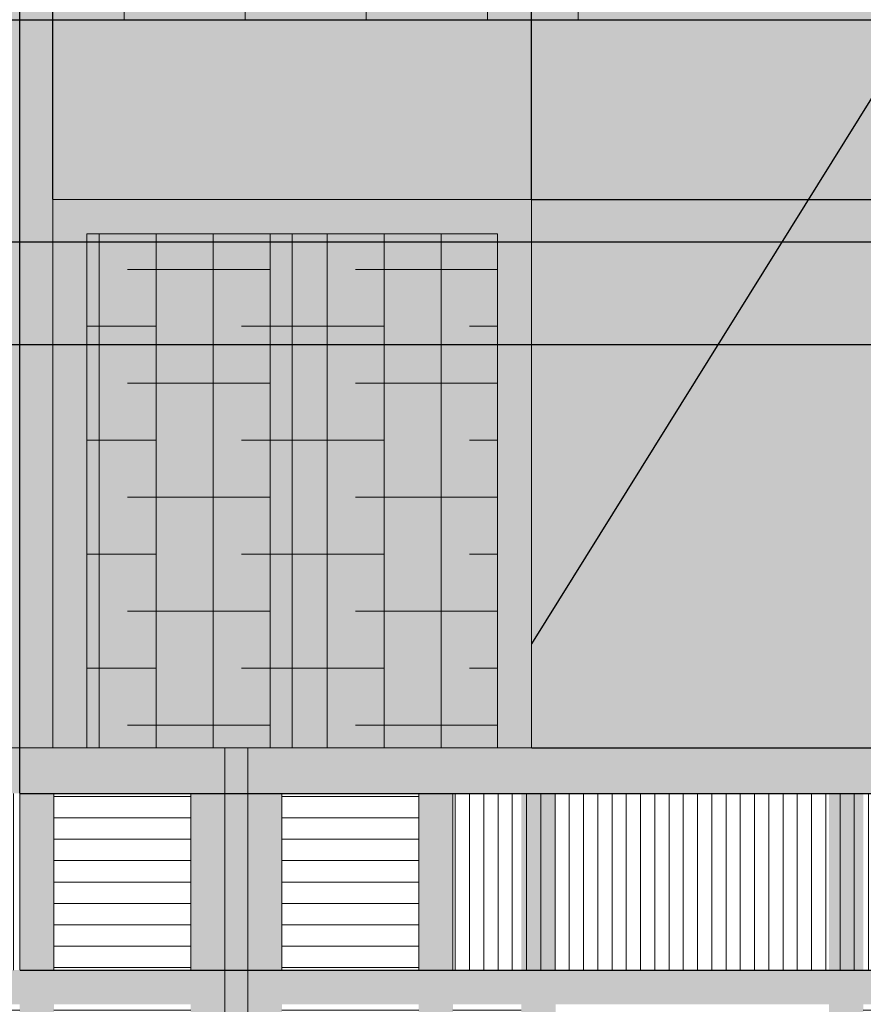
# Model space of a CAD drawing. Units: inches. Extents: x 180 to 1069, y 71 to 1267.
# Tile 4 of 8: x 736 to 884, y 301 to 474. Entities that reach past the tile are written whole.
import ezdxf

# ---------------------------------------------------------------- set-up
doc = ezdxf.new("R2010")
doc.units = ezdxf.units.IN
doc.header["$MEASUREMENT"] = 0
for name, color, linetype, lineweight in [('A-ANNO-DIMS', 2, 'Continuous', 18), ('A-DOOR', 7, 'Continuous', 20), ('A-DOOR-GATE', 7, 'Continuous', 18), ('A-WALL', 7, 'Continuous', 30), ('A-WALL-CLAD', 7, 'Continuous', 18), ('A-WALL-SCRN-JNTS-PATT', 8, 'Continuous', 13)]:
    doc.layers.add(name, color=color, linetype=linetype, lineweight=lineweight)
for name, color, linetype, lineweight, true_color in [('A-DOOR-GATE-PATT', 18, 'Continuous', 13, 0x000000), ('A-DOOR-GLAS-PATT', 152, 'Continuous', 13, 0x2776bb), ('A-DOOR-GRIL-PATT', 177, 'Continuous', 13, 0x293189), ('A-DOOR-HARD-PATT', 8, 'Continuous', 13, 0x7f7f6c), ('A-WALL-PATT', 253, 'Continuous', 13, 0x9f9f8e), ('A-WALL-RCSD-PATT', 251, 'Continuous', 13, 0x696959), ('A-WALL-SCRN-PATT', 251, 'Continuous', 13, 0x636466)]:
    doc.layers.add(name, color=color, linetype=linetype, lineweight=lineweight, true_color=true_color)
doc.styles.get("Standard").update_dxf_attribs({"font": 'arial.ttf'})
doc.dimstyles.get("Standard").update_dxf_attribs({"dimtxt": 6, "dimasz": 2, "dimexe": 0.18, "dimexo": 0.0625, "dimgap": 3, "dimtad": 0, "dimtih": 1, "dimtoh": 1, "dimdec": 0, "dimzin": 0, "dimdsep": 46, "dimlunit": 3, "dimtxsty": 'Standard', "dimcen": 0.09, "dimadec": 0, "dimazin": 0, "dimtfac": 1, "dimtdec": 0, "dimtofl": 0, "dimtmove": 0, "dimatfit": 3, "dimfxl": 1, "dimtolj": 1, "dimtzin": 0, "dimarcsym": 0})

# ---------------------------------------------------------------- blocks, each defined once
blk = doc.blocks.new('*D31')
at = {"layer": 'A-ANNO-DIMS', "color": 0, "lineweight": -2, "transparency": 16777216}
for p, q in [((546.15, 416.82), (1056.28, 416.82)), ((1056.1, 414.82), (1056.1, 278.88)), ((1056.1, 130.82), (1056.1, 266.75)), ((546.15, 128.82), (1056.28, 128.82))]:
    blk.add_line(p, q, dxfattribs=at)
at = {"layer": 'A-ANNO-DIMS', "color": 0, "transparency": 16777216}
for points in [[(1055.77, 414.82), (1056.43, 414.82), (1056.1, 416.82)], [(1055.77, 130.82), (1056.43, 130.82), (1056.1, 128.82)]]:
    blk.add_solid(points, dxfattribs=at)
at = {"layer": 'Defpoints', "color": 0, "transparency": 16777216}
for p in [(546.09, 416.82), (1056.1, 416.82), (546.09, 128.82)]:
    blk.add_point(p, dxfattribs=at)
at = {"layer": 'A-ANNO-DIMS', "color": 0, "transparency": 16777216, "insert": (1056.1, 272.82), "char_height": 6, "attachment_point": 5}
blk.add_mtext('\\A1;288', dxfattribs=at)
blk = doc.blocks.new('*D32')
at = {"layer": 'A-ANNO-DIMS', "color": 0, "lineweight": -2, "transparency": 16777216}
for p, q in [((1056.1, 436.82), (1056.1, 438.82)), ((606.15, 434.82), (1056.28, 434.82)), ((546.15, 416.82), (1056.28, 416.82)), ((1056.1, 414.82), (1056.1, 412.82))]:
    blk.add_line(p, q, dxfattribs=at)
at = {"layer": 'A-ANNO-DIMS', "color": 0, "transparency": 16777216}
for points in [[(1055.77, 436.82), (1056.43, 436.82), (1056.1, 434.82)], [(1055.77, 414.82), (1056.43, 414.82), (1056.1, 416.82)]]:
    blk.add_solid(points, dxfattribs=at)
at = {"layer": 'Defpoints', "color": 0, "transparency": 16777216}
for p in [(606.09, 434.82), (1056.1, 434.82), (546.09, 416.82)]:
    blk.add_point(p, dxfattribs=at)
at = {"layer": 'A-ANNO-DIMS', "color": 0, "transparency": 16777216, "insert": (1056.1, 425.82), "char_height": 6, "attachment_point": 5}
blk.add_mtext('\\A1;18', dxfattribs=at)
blk = doc.blocks.new('*D40')
at = {"layer": 'A-ANNO-DIMS', "color": 0, "lineweight": -2, "transparency": 16777216}
for p, q in [((652.09, 338.11), (652.09, 1263.01)), ((736.09, 338.11), (736.09, 1263.01)), ((654.09, 1262.83), (686.8, 1262.83)), ((734.09, 1262.83), (701.38, 1262.83))]:
    blk.add_line(p, q, dxfattribs=at)
at = {"layer": 'A-ANNO-DIMS', "color": 0, "transparency": 16777216}
for points in [[(654.09, 1263.16), (654.09, 1262.5), (652.09, 1262.83)], [(734.09, 1263.16), (734.09, 1262.5), (736.09, 1262.83)]]:
    blk.add_solid(points, dxfattribs=at)
at = {"layer": 'Defpoints', "color": 0, "transparency": 16777216}
for p in [(736.09, 1262.83), (652.09, 338.05), (736.09, 338.05)]:
    blk.add_point(p, dxfattribs=at)
at = {"layer": 'A-ANNO-DIMS', "color": 0, "transparency": 16777216, "insert": (694.09, 1262.83), "char_height": 6, "attachment_point": 5}
blk.add_mtext('\\A1;84', dxfattribs=at)
blk = doc.blocks.new('*D41')
at = {"layer": 'A-ANNO-DIMS', "color": 0, "lineweight": -2, "transparency": 16777216}
for p, q in [((736.15, 338.05), (1056.28, 338.05)), ((1056.1, 336.05), (1056.1, 328.61)), ((1056.1, 309.05), (1056.1, 316.48)), ((736.15, 307.05), (1056.28, 307.05))]:
    blk.add_line(p, q, dxfattribs=at)
at = {"layer": 'A-ANNO-DIMS', "color": 0, "transparency": 16777216}
for points in [[(1055.77, 336.05), (1056.43, 336.05), (1056.1, 338.05)], [(1055.77, 309.05), (1056.43, 309.05), (1056.1, 307.05)]]:
    blk.add_solid(points, dxfattribs=at)
at = {"layer": 'Defpoints', "color": 0, "transparency": 16777216}
for p in [(736.09, 338.05), (736.09, 307.05), (1056.1, 307.05)]:
    blk.add_point(p, dxfattribs=at)
at = {"layer": 'A-ANNO-DIMS', "color": 0, "transparency": 16777216, "insert": (1056.1, 322.55), "char_height": 6, "attachment_point": 5}
blk.add_mtext('\\A1;31', dxfattribs=at)
blk = doc.blocks.new('*D45')
at = {"layer": 'A-ANNO-DIMS', "color": 0, "lineweight": -2, "transparency": 16777216}
for p, q in [((690, 442.3), (690, 1263.01)), ((741.89, 442.3), (741.89, 1263.01)), ((692, 1262.83), (702.82, 1262.83)), ((739.89, 1262.83), (729.08, 1262.83))]:
    blk.add_line(p, q, dxfattribs=at)
at = {"layer": 'A-ANNO-DIMS', "color": 0, "transparency": 16777216}
for points in [[(692, 1263.16), (692, 1262.5), (690, 1262.83)], [(739.89, 1263.16), (739.89, 1262.5), (741.89, 1262.83)]]:
    blk.add_solid(points, dxfattribs=at)
at = {"layer": 'Defpoints', "color": 0, "transparency": 16777216}
for p in [(741.89, 1262.83), (690, 442.24), (741.89, 442.24)]:
    blk.add_point(p, dxfattribs=at)
at = {"layer": 'A-ANNO-DIMS', "color": 0, "transparency": 16777216, "insert": (715.95, 1262.83), "char_height": 6, "attachment_point": 5}
blk.add_mtext('\\A1;51.89', dxfattribs=at)
blk = doc.blocks.new('*D46')
at = {"layer": 'A-ANNO-DIMS', "color": 0, "lineweight": -2, "transparency": 16777216}
for p, q in [((741.89, 442.3), (741.89, 1263.01)), ((825.89, 442.3), (825.89, 1263.01)), ((743.89, 1262.83), (776.6, 1262.83)), ((823.89, 1262.83), (791.18, 1262.83))]:
    blk.add_line(p, q, dxfattribs=at)
at = {"layer": 'A-ANNO-DIMS', "color": 0, "transparency": 16777216}
for points in [[(743.89, 1263.16), (743.89, 1262.5), (741.89, 1262.83)], [(823.89, 1263.16), (823.89, 1262.5), (825.89, 1262.83)]]:
    blk.add_solid(points, dxfattribs=at)
at = {"layer": 'Defpoints', "color": 0, "transparency": 16777216}
for p in [(825.89, 1262.83), (741.89, 442.24), (825.89, 442.24)]:
    blk.add_point(p, dxfattribs=at)
at = {"layer": 'A-ANNO-DIMS', "color": 0, "transparency": 16777216, "insert": (783.89, 1262.83), "char_height": 6, "attachment_point": 5}
blk.add_mtext('\\A1;84', dxfattribs=at)
blk = doc.blocks.new('*D47')
at = {"layer": 'A-ANNO-DIMS', "color": 0, "lineweight": -2, "transparency": 16777216}
for p, q in [((825.96, 442.24), (1056.28, 442.24)), ((1056.1, 440.24), (1056.1, 400.21)), ((1056.1, 348.05), (1056.1, 388.08)), ((825.96, 346.05), (1056.28, 346.05))]:
    blk.add_line(p, q, dxfattribs=at)
at = {"layer": 'A-ANNO-DIMS', "color": 0, "transparency": 16777216}
for points in [[(1055.77, 440.24), (1056.43, 440.24), (1056.1, 442.24)], [(1055.77, 348.05), (1056.43, 348.05), (1056.1, 346.05)]]:
    blk.add_solid(points, dxfattribs=at)
at = {"layer": 'Defpoints', "color": 0, "transparency": 16777216}
for p in [(825.89, 442.24), (1056.1, 442.24), (825.89, 346.05)]:
    blk.add_point(p, dxfattribs=at)
at = {"layer": 'A-ANNO-DIMS', "color": 0, "transparency": 16777216, "insert": (1056.1, 394.14), "char_height": 6, "attachment_point": 5}
blk.add_mtext('\\A1;96.2', dxfattribs=at)
blk = doc.blocks.new('*D59')
at = {"layer": 'A-ANNO-DIMS', "color": 0, "lineweight": -2, "transparency": 16777216}
for p, q in [((606.15, 1010.82), (1056.28, 1010.82)), ((1056.1, 1008.82), (1056.1, 728.88)), ((1056.1, 436.82), (1056.1, 716.75)), ((606.15, 434.82), (1056.28, 434.82))]:
    blk.add_line(p, q, dxfattribs=at)
at = {"layer": 'A-ANNO-DIMS', "color": 0, "transparency": 16777216}
for points in [[(1055.77, 1008.82), (1056.43, 1008.82), (1056.1, 1010.82)], [(1055.77, 436.82), (1056.43, 436.82), (1056.1, 434.82)]]:
    blk.add_solid(points, dxfattribs=at)
at = {"layer": 'Defpoints', "color": 0, "transparency": 16777216}
for p in [(606.09, 1010.82), (1056.1, 1010.82), (606.09, 434.82)]:
    blk.add_point(p, dxfattribs=at)
at = {"layer": 'A-ANNO-DIMS', "color": 0, "transparency": 16777216, "insert": (1056.1, 722.82), "char_height": 6, "attachment_point": 5}
blk.add_mtext('\\A1;576', dxfattribs=at)
blk = doc.blocks.new('*D60')
at = {"layer": 'A-ANNO-DIMS', "color": 0, "lineweight": -2, "transparency": 16777216}
for p, q in [((498.15, 488.82), (1056.28, 488.82)), ((1056.1, 486.82), (1056.1, 467.87)), ((1056.1, 436.82), (1056.1, 455.76)), ((606.15, 434.82), (1056.28, 434.82))]:
    blk.add_line(p, q, dxfattribs=at)
at = {"layer": 'A-ANNO-DIMS', "color": 0, "transparency": 16777216}
for points in [[(1055.77, 486.82), (1056.43, 486.82), (1056.1, 488.82)], [(1055.77, 436.82), (1056.43, 436.82), (1056.1, 434.82)]]:
    blk.add_solid(points, dxfattribs=at)
at = {"layer": 'Defpoints', "color": 0, "transparency": 16777216}
for p in [(498.09, 488.82), (606.09, 434.82), (1056.1, 434.82)]:
    blk.add_point(p, dxfattribs=at)
at = {"layer": 'A-ANNO-DIMS', "color": 0, "transparency": 16777216, "insert": (1056.1, 461.82), "char_height": 6, "attachment_point": 5}
blk.add_mtext('\\A1;54', dxfattribs=at)
blk = doc.blocks.new('*D68')
at = {"layer": 'A-ANNO-DIMS', "color": 0, "lineweight": -2, "transparency": 16777216}
for p, q in [((702.09, 557.75), (702.09, 74.62)), ((1002.09, 557.75), (1002.09, 74.62)), ((704.09, 74.8), (842.47, 74.8)), ((1000.09, 74.8), (861.7, 74.8))]:
    blk.add_line(p, q, dxfattribs=at)
at = {"layer": 'A-ANNO-DIMS', "color": 0, "transparency": 16777216}
for points in [[(704.09, 75.14), (704.09, 74.47), (702.09, 74.8)], [(1000.09, 75.14), (1000.09, 74.47), (1002.09, 74.8)]]:
    blk.add_solid(points, dxfattribs=at)
at = {"layer": 'Defpoints', "color": 0, "transparency": 16777216}
for p in [(702.09, 557.82), (1002.09, 557.82), (1002.09, 74.8)]:
    blk.add_point(p, dxfattribs=at)
at = {"layer": 'A-ANNO-DIMS', "color": 0, "transparency": 16777216, "insert": (852.09, 74.8), "char_height": 6, "attachment_point": 5}
blk.add_mtext('\\A1;300', dxfattribs=at)

msp = doc.modelspace()

# ---------------------------------------------------------------- hatches: boundary and pattern name
at = {"layer": 'A-DOOR-GATE-PATT'}
h = msp.add_hatch(color=256, dxfattribs=at)
h.dxf.hatch_style = 1
h.paths.add_polyline_path([(772.0875, 346.0477), (630.0875, 346.0477), (630.0875, 338.0477), (646.0875, 338.0477), (646.0875, 307.0477), (630.0875, 307.0477), (630.0875, 301.0477), (646.0875, 301.0477), (646.0875, 276.8159), (630.0875, 276.8159), (630.0875, 270.8159), (646.0875, 270.8159), (646.0875, 246.8159), (630.0875, 246.8159), (630.0875, 240.8159), (646.0875, 240.8159), (646.0875, 216.8159), (630.0875, 216.8159), (630.0875, 210.8159), (646.0875, 210.8159), (646.0875, 186.8159), (630.0875, 186.8159), (630.0875, 178.8159), (766.0875, 178.8159), (766.0875, 148.8159), (630.0875, 148.8159), (630.0875, 140.8159), (772.0875, 140.8159)])
h.paths.add_polyline_path([(670.0875, 338.0477), (718.0875, 338.0477), (718.0875, 307.0477), (670.0875, 307.0477)], flags=16)
h.paths.add_polyline_path([(664.0875, 338.0477), (664.0875, 307.0477), (652.0875, 307.0477), (652.0875, 338.0477)], flags=16)
h.paths.add_polyline_path([(670.0875, 301.0477), (718.0875, 301.0477), (718.0875, 276.8159), (670.0875, 276.8159)], flags=16)
h.paths.add_polyline_path([(664.0875, 301.0477), (664.0875, 276.8159), (652.0875, 276.8159), (652.0875, 301.0477)], flags=16)
h.paths.add_polyline_path([(724.0875, 338.0477), (736.0875, 338.0477), (736.0875, 307.0477), (724.0875, 307.0477)], flags=16)
h.paths.add_polyline_path([(724.0875, 301.0477), (736.0875, 301.0477), (736.0875, 276.8159), (724.0875, 276.8159)], flags=16)
h.paths.add_polyline_path([(670.0875, 270.8159), (718.0875, 270.8159), (718.0875, 246.8159), (670.0875, 246.8159)], flags=16)
h.paths.add_polyline_path([(664.0875, 270.8159), (664.0875, 246.8159), (652.0875, 246.8159), (652.0875, 270.8159)], flags=16)
h.paths.add_polyline_path([(742.0875, 338.0477), (766.0875, 338.0477), (766.0875, 307.0477), (742.0875, 307.0477)], flags=16)
h.paths.add_polyline_path([(742.0875, 301.0477), (766.0875, 301.0477), (766.0875, 276.8159), (742.0875, 276.8159)], flags=16)
h.paths.add_polyline_path([(724.0875, 270.8159), (736.0875, 270.8159), (736.0875, 246.8159), (724.0875, 246.8159)], flags=16)
h.paths.add_polyline_path([(670.0875, 240.8159), (718.0875, 240.8159), (718.0875, 216.8159), (670.0875, 216.8159)], flags=16)
h.paths.add_polyline_path([(664.0875, 240.8159), (664.0875, 216.8159), (652.0875, 216.8159), (652.0875, 240.8159)], flags=16)
h.paths.add_polyline_path([(742.0875, 270.8159), (766.0875, 270.8159), (766.0875, 246.8159), (742.0875, 246.8159)], flags=16)
h.paths.add_polyline_path([(724.0875, 240.8159), (736.0875, 240.8159), (736.0875, 216.8159), (724.0875, 216.8159)], flags=16)
h.paths.add_polyline_path([(742.0875, 240.8159), (766.0875, 240.8159), (766.0875, 216.8159), (742.0875, 216.8159)], flags=16)
h.paths.add_polyline_path([(670.0875, 210.8159), (718.0875, 210.8159), (718.0875, 186.8159), (670.0875, 186.8159)], flags=16)
h.paths.add_polyline_path([(664.0875, 210.8159), (664.0875, 186.8159), (652.0875, 186.8159), (652.0875, 210.8159)], flags=16)
h.paths.add_polyline_path([(724.0875, 210.8159), (736.0875, 210.8159), (736.0875, 186.8159), (724.0875, 186.8159)], flags=16)
h.paths.add_polyline_path([(742.0875, 210.8159), (766.0875, 210.8159), (766.0875, 186.8159), (742.0875, 186.8159)], flags=16)
h.paths.add_polyline_path([(918.0875, 346.0477), (776.0875, 346.0477), (776.0875, 140.8159), (918.0875, 140.8159), (918.0875, 148.8159), (782.0875, 148.8159), (782.0875, 178.8159), (918.0875, 178.8159), (918.0875, 186.8159), (902.0875, 186.8159), (902.0875, 210.8159), (918.0875, 210.8159), (918.0875, 216.8159), (902.0875, 216.8159), (902.0875, 240.8159), (918.0875, 240.8159), (918.0875, 246.8159), (902.0875, 246.8159), (902.0875, 270.8159), (918.0875, 270.8159), (918.0875, 276.8159), (902.0875, 276.8159), (902.0875, 301.0477), (918.0875, 301.0477), (918.0875, 307.0477), (902.0875, 307.0477), (902.0875, 338.0477), (918.0875, 338.0477)])
h.paths.add_polyline_path([(782.0875, 338.0477), (806.0875, 338.0477), (806.0875, 307.0477), (782.0875, 307.0477)], flags=16)
h.paths.add_polyline_path([(812.0875, 338.0477), (824.0875, 338.0477), (824.0875, 307.0477), (812.0875, 307.0477)], flags=16)
h.paths.add_polyline_path([(782.0875, 301.0477), (806.0875, 301.0477), (806.0875, 276.8159), (782.0875, 276.8159)], flags=16)
h.paths.add_polyline_path([(830.0875, 338.0477), (878.0875, 338.0477), (878.0875, 307.0477), (830.0875, 307.0477)], flags=16)
h.paths.add_polyline_path([(812.0875, 301.0477), (824.0875, 301.0477), (824.0875, 276.8159), (812.0875, 276.8159)], flags=16)
h.paths.add_polyline_path([(830.0875, 301.0477), (878.0875, 301.0477), (878.0875, 276.8159), (830.0875, 276.8159)], flags=16)
h.paths.add_polyline_path([(782.0875, 270.8159), (806.0875, 270.8159), (806.0875, 246.8159), (782.0875, 246.8159)], flags=16)
h.paths.add_polyline_path([(812.0875, 270.8159), (824.0875, 270.8159), (824.0875, 246.8159), (812.0875, 246.8159)], flags=16)
h.paths.add_polyline_path([(830.0875, 270.8159), (878.0875, 270.8159), (878.0875, 246.8159), (830.0875, 246.8159)], flags=16)
h.paths.add_polyline_path([(782.0875, 240.8159), (806.0875, 240.8159), (806.0875, 216.8159), (782.0875, 216.8159)], flags=16)
h.paths.add_polyline_path([(884.0875, 338.0477), (896.0875, 338.0477), (896.0875, 307.0477), (884.0875, 307.0477)], flags=16)
h.paths.add_polyline_path([(812.0875, 240.8159), (824.0875, 240.8159), (824.0875, 216.8159), (812.0875, 216.8159)], flags=16)
h.paths.add_polyline_path([(884.0875, 301.0477), (896.0875, 301.0477), (896.0875, 276.8159), (884.0875, 276.8159)], flags=16)
h.paths.add_polyline_path([(830.0875, 240.8159), (878.0875, 240.8159), (878.0875, 216.8159), (830.0875, 216.8159)], flags=16)
h.paths.add_polyline_path([(884.0875, 270.8159), (896.0875, 270.8159), (896.0875, 246.8159), (884.0875, 246.8159)], flags=16)
h.paths.add_polyline_path([(782.0875, 210.8159), (806.0875, 210.8159), (806.0875, 186.8159), (782.0875, 186.8159)], flags=16)
h.paths.add_polyline_path([(812.0875, 210.8159), (824.0875, 210.8159), (824.0875, 186.8159), (812.0875, 186.8159)], flags=16)
h.paths.add_polyline_path([(830.0875, 210.8159), (878.0875, 210.8159), (878.0875, 186.8159), (830.0875, 186.8159)], flags=16)
h.paths.add_polyline_path([(884.0875, 240.8159), (896.0875, 240.8159), (896.0875, 216.8159), (884.0875, 216.8159)], flags=16)
h.paths.add_polyline_path([(884.0875, 210.8159), (896.0875, 210.8159), (896.0875, 186.8159), (884.0875, 186.8159)], flags=16)
h = msp.add_hatch(dxfattribs=at)
h.set_pattern_fill('ANSI31', color=256, scale=30, angle=135)
h.paths.add_polyline_path([(646.0875, 338.0477), (630.0875, 338.0477), (630.0875, 307.0477), (646.0875, 307.0477)])
h.paths.add_polyline_path([(646.0875, 301.0477), (630.0875, 301.0477), (630.0875, 276.8159), (646.0875, 276.8159)])
h.paths.add_polyline_path([(664.0875, 301.0477), (652.0875, 301.0477), (652.0875, 276.8159), (664.0875, 276.8159)])
h.paths.add_polyline_path([(664.0875, 270.8159), (652.0875, 270.8159), (652.0875, 246.8159), (664.0875, 246.8159)])
h.paths.add_polyline_path([(646.0875, 270.8159), (630.0875, 270.8159), (630.0875, 246.8159), (646.0875, 246.8159)])
h.paths.add_polyline_path([(646.0875, 240.8159), (630.0875, 240.8159), (630.0875, 216.8159), (646.0875, 216.8159)])
h.paths.add_polyline_path([(664.0875, 240.8159), (652.0875, 240.8159), (652.0875, 216.8159), (664.0875, 216.8159)])
h.paths.add_polyline_path([(664.0875, 210.8159), (652.0875, 210.8159), (652.0875, 186.8159), (664.0875, 186.8159)])
h.paths.add_polyline_path([(646.0875, 210.8159), (630.0875, 210.8159), (630.0875, 186.8159), (646.0875, 186.8159)])
h.paths.add_polyline_path([(736.0875, 301.0477), (724.0875, 301.0477), (724.0875, 276.8159), (736.0875, 276.8159)])
h.paths.add_polyline_path([(766.0875, 301.0477), (742.0875, 301.0477), (742.0875, 276.8159), (766.0875, 276.8159)])
h.paths.add_polyline_path([(766.0875, 270.8159), (742.0875, 270.8159), (742.0875, 246.8159), (766.0875, 246.8159)])
h.paths.add_polyline_path([(766.0875, 338.0477), (742.0875, 338.0477), (742.0875, 307.0477), (766.0875, 307.0477)])
h.paths.add_polyline_path([(736.0875, 270.8159), (724.0875, 270.8159), (724.0875, 246.8159), (736.0875, 246.8159)])
h.paths.add_polyline_path([(736.0875, 240.8159), (724.0875, 240.8159), (724.0875, 216.8159), (736.0875, 216.8159)])
h.paths.add_polyline_path([(766.0875, 240.8159), (742.0875, 240.8159), (742.0875, 216.8159), (766.0875, 216.8159)])
h.paths.add_polyline_path([(766.0875, 210.8159), (742.0875, 210.8159), (742.0875, 186.8159), (766.0875, 186.8159)])
h.paths.add_polyline_path([(736.0875, 210.8159), (724.0875, 210.8159), (724.0875, 186.8159), (736.0875, 186.8159)])
h.paths.add_polyline_path([(806.0875, 210.8159), (782.0875, 210.8159), (782.0875, 186.8159), (806.0875, 186.8159)])
h.paths.add_polyline_path([(806.0875, 240.8159), (782.0875, 240.8159), (782.0875, 216.8159), (806.0875, 216.8159)])
h.paths.add_polyline_path([(806.0875, 270.8159), (782.0875, 270.8159), (782.0875, 246.8159), (806.0875, 246.8159)])
h.paths.add_polyline_path([(806.0875, 301.0477), (782.0875, 301.0477), (782.0875, 276.8159), (806.0875, 276.8159)])
h.paths.add_polyline_path([(806.0875, 338.0477), (782.0875, 338.0477), (782.0875, 307.0477), (806.0875, 307.0477)])
h.paths.add_polyline_path([(824.0875, 301.0477), (812.0875, 301.0477), (812.0875, 276.8159), (824.0875, 276.8159)])
h.paths.add_polyline_path([(824.0875, 270.8159), (812.0875, 270.8159), (812.0875, 246.8159), (824.0875, 246.8159)])
h.paths.add_polyline_path([(824.0875, 240.8159), (812.0875, 240.8159), (812.0875, 216.8159), (824.0875, 216.8159)])
h.paths.add_polyline_path([(824.0875, 210.8159), (812.0875, 210.8159), (812.0875, 186.8159), (824.0875, 186.8159)])
h.paths.add_polyline_path([(918.0875, 338.0477), (902.0875, 338.0477), (902.0875, 307.0477), (918.0875, 307.0477)])
h.paths.add_polyline_path([(918.0875, 301.0477), (902.0875, 301.0477), (902.0875, 276.8159), (918.0875, 276.8159)])
h.paths.add_polyline_path([(918.0875, 270.8159), (902.0875, 270.8159), (902.0875, 246.8159), (918.0875, 246.8159)])
h.paths.add_polyline_path([(918.0875, 240.8159), (902.0875, 240.8159), (902.0875, 216.8159), (918.0875, 216.8159)])
h.paths.add_polyline_path([(918.0875, 210.8159), (902.0875, 210.8159), (902.0875, 186.8159), (918.0875, 186.8159)])
h.paths.add_polyline_path([(896.0875, 210.8159), (884.0875, 210.8159), (884.0875, 186.8159), (896.0875, 186.8159)])
h.paths.add_polyline_path([(896.0875, 240.8159), (884.0875, 240.8159), (884.0875, 216.8159), (896.0875, 216.8159)])
h.paths.add_polyline_path([(896.0875, 270.8159), (884.0875, 270.8159), (884.0875, 246.8159), (896.0875, 246.8159)])
h.paths.add_polyline_path([(896.0875, 301.0477), (884.0875, 301.0477), (884.0875, 276.8159), (896.0875, 276.8159)])
h = msp.add_hatch(dxfattribs=at)
h.set_pattern_fill('ANSI31', color=256, scale=20, angle=45)
h.paths.add_polyline_path([(736.0875, 338.0477), (724.0875, 338.0477), (664.0875, 338.0477), (652.0875, 338.0477), (652.0875, 307.0477), (664.0875, 307.0477), (724.0875, 307.0477), (736.0875, 307.0477)])
h.paths.add_polyline_path([(896.0875, 338.0477), (884.0875, 338.0477), (824.0875, 338.0477), (812.0875, 338.0477), (812.0875, 307.0477), (830.0875, 307.0477), (884.0875, 307.0477), (896.0875, 307.0477)])
at = {"layer": 'A-DOOR-GLAS-PATT'}
h = msp.add_hatch(color=256, dxfattribs=at)
h.dxf.hatch_style = 1
h.paths.add_polyline_path([(783.8928, 436.2382), (747.8928, 436.2382), (747.8928, 346.0477), (776.0875, 346.0477), (783.8928, 346.0477)], flags=17)
h.paths.add_polyline_path([(819.8928, 436.2382), (783.8928, 436.2382), (783.8928, 346.0477), (819.8928, 346.0477)], flags=17)
at = {"layer": 'A-DOOR-GRIL-PATT'}
h = msp.add_hatch(color=256, dxfattribs=at)
h.dxf.hatch_style = 1
h.paths.add_polyline_path([(825.8928, 442.2382), (741.8928, 442.2382), (741.8928, 346.0477), (747.8928, 346.0477), (747.8928, 436.2382), (819.8928, 436.2382), (819.8928, 346.0477), (825.8928, 346.0477)])
h = msp.add_hatch(dxfattribs=at)
h.set_pattern_fill('ANSI38', color=256, scale=80, angle=45)
h.paths.add_polyline_path([(783.8928, 436.2382), (747.8928, 436.2382), (747.8928, 346.0477), (776.0875, 346.0477), (783.8928, 346.0477)])
h = msp.add_hatch(dxfattribs=at)
h.set_pattern_fill('ANSI38', color=256, scale=80, angle=45)
h.paths.add_polyline_path([(819.8928, 436.2382), (783.8928, 436.2382), (783.8928, 346.0477), (819.8928, 346.0477)])
at = {"layer": 'A-DOOR-HARD-PATT'}
h = msp.add_hatch(color=256, dxfattribs=at)
h.dxf.hatch_style = 1
h.paths.add_polyline_path([(776.0875, 346.0477), (772.0875, 346.0477), (772.0875, 140.8159), (776.0875, 140.8159)])
at = {"layer": 'A-WALL-PATT'}
h = msp.add_hatch(color=256, dxfattribs=at)
h.dxf.hatch_style = 1
h.paths.add_polyline_path([(978.0875, 947.2513), (834.0875, 947.2513), (834.0875, 869.8159), (978.0875, 869.8159)])
h.paths.add_polyline_path([(978.0875, 557.8159), (834.0875, 557.8159), (834.0875, 473.8159), (978.0875, 473.8159)])
h.paths.add_polyline_path([(960.2423, 791.8159), (606.0875, 791.8159), (606.0875, 647.8159), (883.3511, 647.8159), (883.3511, 731.8159), (907.3511, 731.8159)])
h = msp.add_hatch(color=256, dxfattribs=at)
h.dxf.hatch_style = 1
h.paths.add_polyline_path([(894.0875, 473.8159), (825.8928, 364.2866), (825.8928, 346.0477), (894.0875, 346.0477)])
at = {"layer": 'A-WALL-RCSD-PATT'}
h = msp.add_hatch(color=256, dxfattribs=at)
h.dxf.hatch_style = 1
h.paths.add_polyline_path([(741.8928, 442.2382), (825.8928, 442.2382), (825.8928, 364.2866), (894.0875, 473.8159), (606.0875, 473.8159), (606.0875, 442.2382), (690.001, 442.2382), (690.001, 346.0477), (741.8928, 346.0477)])
at = {"layer": 'A-WALL-SCRN-JNTS-PATT'}
h = msp.add_hatch(dxfattribs=at)
h.set_pattern_fill('ANSI36', color=256, scale=85, angle=45)
h.paths.add_polyline_path([(606.0875, 938.8159), (798.0875, 938.8159), (798.0875, 869.8159), (834.0875, 869.8159), (834.0875, 974.8159), (606.0875, 974.8159), (606.0875, 1010.8159), (354.0875, 1010.8159), (354.0875, 984.0304), (467.1892, 984.0304), (467.1892, 956.8159), (498.0875, 956.8159), (498.0875, 488.8159), (467.1892, 488.8159), (467.1892, 456.1177), (354.0875, 456.1177), (354.0875, 434.8159), (606.0875, 434.8159), (606.0875, 473.8159), (834.0875, 473.8159), (834.0875, 557.8159), (798.0875, 557.8159), (798.0875, 509.8159), (606.0875, 509.8159)])
at = {"layer": 'A-WALL-SCRN-PATT'}
h = msp.add_hatch(color=256, dxfattribs=at)
h.dxf.hatch_style = 1
h.paths.add_polyline_path([(606.0875, 938.8159), (798.0875, 938.8159), (798.0875, 869.8159), (834.0875, 869.8159), (834.0875, 974.8159), (606.0875, 974.8159), (606.0875, 1010.8159), (354.0875, 1010.8159), (354.0875, 984.0304), (467.1892, 984.0304), (467.1892, 956.8159), (498.0875, 956.8159), (498.0875, 488.8159), (467.1892, 488.8159), (467.1892, 456.1177), (354.0875, 456.1177), (354.0875, 434.8159), (606.0875, 434.8159), (606.0875, 473.8159), (834.0875, 473.8159), (834.0875, 557.8159), (798.0875, 557.8159), (798.0875, 509.8159), (606.0875, 509.8159)])
h.paths.add_polyline_path([(367.1892, 507.1177), (326.1892, 507.1177), (326.1892, 465.1177), (367.1892, 465.1177)])
h.paths.add_polyline_path([(411.1892, 507.1177), (373.1892, 507.1177), (373.1892, 465.1177), (411.1892, 465.1177)], flags=17)
h.paths.add_polyline_path([(458.1892, 507.1177), (417.1892, 507.1177), (417.1892, 465.1177), (458.1892, 465.1177)], flags=17)
h.paths.add_polyline_path([(426.0875, 672.0741), (354.0875, 672.0741), (354.0875, 636.0741), (426.0875, 636.0741)], flags=17)
h.paths.add_polyline_path([(426.0875, 760.0741), (354.0875, 760.0741), (354.0875, 680.0741), (426.0875, 680.0741)], flags=17)
h.paths.add_polyline_path([(426.0875, 804.0741), (354.0875, 804.0741), (354.0875, 768.0741), (426.0875, 768.0741)], flags=17)
h.paths.add_polyline_path([(367.1892, 975.0304), (326.1892, 975.0304), (326.1892, 933.0304), (367.1892, 933.0304)])
h.paths.add_polyline_path([(411.1892, 975.0304), (373.1892, 975.0304), (373.1892, 933.0304), (411.1892, 933.0304)], flags=17)
h.paths.add_polyline_path([(458.1892, 975.0304), (417.1892, 975.0304), (417.1892, 933.0304), (458.1892, 933.0304)], flags=17)

# ---------------------------------------------------------------- linework, layer by layer
at = {"layer": 'A-DOOR'}
for p, q in [((741.8928, 346.0477), (741.8928, 442.2382)), ((741.8928, 442.2382), (825.8928, 442.2382)), ((825.8928, 442.2382), (825.8928, 346.0477)), ((747.8928, 346.0477), (747.8928, 436.2382)), ((747.8928, 436.2382), (819.8928, 436.2382)), ((783.8928, 436.2382), (783.8928, 346.0477)), ((819.8928, 436.2382), (819.8928, 346.0477))]:
    msp.add_line(p, q, dxfattribs=at)
at = {"layer": 'A-DOOR-GATE'}
for p, q in [((630.0875, 346.0477), (776.0875, 346.0477)), ((772.0875, 346.0477), (772.0875, 140.8159)), ((776.0875, 346.0477), (776.0875, 140.8159)), ((776.0875, 346.0477), (918.0875, 346.0477)), ((736.0875, 338.0477), (736.0875, 307.0477)), ((742.0875, 338.0477), (742.0875, 307.0477)), ((742.0875, 338.0477), (766.0875, 338.0477)), ((766.0875, 338.0477), (766.0875, 307.0477)), ((782.0875, 338.0477), (782.0875, 307.0477)), ((782.0875, 338.0477), (806.0875, 338.0477)), ((806.0875, 338.0477), (806.0875, 307.0477)), ((812.0875, 338.0477), (812.0875, 307.0477)), ((812.0875, 338.0477), (824.0875, 338.0477)), ((824.0875, 338.0477), (884.0875, 338.0477)), ((884.0875, 338.0477), (896.0875, 338.0477)), ((742.0875, 307.0477), (766.0875, 307.0477)), ((782.0875, 307.0477), (806.0875, 307.0477)), ((812.0875, 307.0477), (830.0875, 307.0477)), ((830.0875, 307.0477), (884.0875, 307.0477)), ((884.0875, 307.0477), (896.0875, 307.0477))]:
    msp.add_line(p, q, dxfattribs=at)
at = {"layer": 'A-WALL'}
for p, q in [((606.0875, 473.8159), (978.0875, 473.8159)), ((894.0875, 473.8159), (825.8928, 364.2866))]:
    msp.add_line(p, q, dxfattribs=at)
at = {"layer": 'A-WALL-CLAD'}
msp.add_line((834.0875, 557.8159), (834.0875, 473.8159), dxfattribs=at)

# ---------------------------------------------------------------- dimensions: what is measured, and where the dimension line sits
at = {"layer": 'A-ANNO-DIMS'}
for base, p1, p2, override, picture, middle in [((736.0875, 1262.8294), (652.0875, 338.0477), (736.0875, 338.0477), {"dimdec": 0, "dimlfac": 1, "dimrnd": 0, "dimzin": 0, "dimdsep": 46, "dimlunit": 2}, '*D40', (694.0875, 1262.8294)), ((741.8928, 1262.8294), (690.001, 442.2382), (741.8928, 442.2382), {"dimdec": 2, "dimlfac": 1, "dimrnd": 0, "dimzin": 0, "dimdsep": 46, "dimlunit": 2}, '*D45', (715.9469, 1262.8294)), ((825.8928, 1262.8294), (741.8928, 442.2382), (825.8928, 442.2382), {"dimdec": 0, "dimlfac": 1, "dimrnd": 0, "dimzin": 0, "dimdsep": 46, "dimlunit": 2}, '*D46', (783.8928, 1262.8294)), ((1002.0875, 74.8024), (702.0875, 557.8159), (1002.0875, 557.8159), {"dimdec": 0, "dimlfac": 1, "dimrnd": 0, "dimzin": 0, "dimdsep": 46, "dimlunit": 2}, '*D68', (852.0875, 74.8024))]:
    dim = msp.add_linear_dim(base=base, p1=p1, p2=p2, dimstyle='Standard', override=override, dxfattribs=at)
    dim.commit()
    dim.dimension.update_dxf_attribs({"geometry": picture, "text_midpoint": middle})
for base, p1, p2, override, picture, middle in [((1056.101, 1010.8159), (606.0875, 434.8159), (606.0875, 1010.8159), {"dimdec": 0, "dimlfac": 1, "dimrnd": 0, "dimzin": 0, "dimdsep": 46, "dimlunit": 2}, '*D59', (1056.101, 722.8159)), ((1056.101, 434.8159), (498.0875, 488.8159), (606.0875, 434.8159), {"dimdec": 0, "dimlfac": 1, "dimrnd": 0, "dimzin": 0, "dimdsep": 46, "dimlunit": 2}, '*D60', (1056.101, 461.8159)), ((1056.101, 442.2382), (825.8928, 346.0477), (825.8928, 442.2382), {"dimdec": 1, "dimlfac": 1, "dimrnd": 0, "dimzin": 0, "dimdsep": 46, "dimlunit": 2}, '*D47', (1056.101, 394.1429)), ((1056.101, 434.8159), (546.0875, 416.8159), (606.0875, 434.8159), {"dimdec": 0, "dimlfac": 1, "dimrnd": 0, "dimzin": 0, "dimdsep": 46, "dimlunit": 2}, '*D32', (1056.101, 425.8159)), ((1056.101, 416.8159), (546.0875, 128.8159), (546.0875, 416.8159), {"dimdec": 0, "dimlfac": 1, "dimrnd": 0, "dimzin": 0, "dimdsep": 46, "dimlunit": 2}, '*D31', (1056.101, 272.8159)), ((1056.101, 307.0477), (736.0875, 338.0477), (736.0875, 307.0477), {"dimdec": 0, "dimlfac": 1, "dimrnd": 0, "dimzin": 0, "dimdsep": 46, "dimlunit": 2}, '*D41', (1056.101, 322.5477))]:
    dim = msp.add_linear_dim(base=base, p1=p1, p2=p2, angle=90, dimstyle='Standard', override=override, dxfattribs=at)
    dim.commit()
    dim.dimension.update_dxf_attribs({"geometry": picture, "text_midpoint": middle})

doc.saveas('drawing.dxf')
